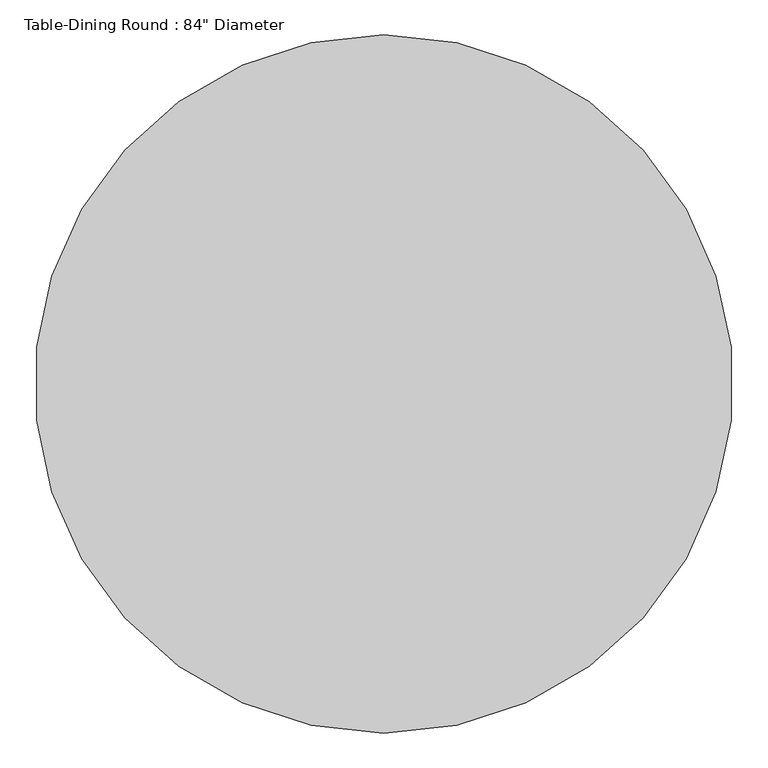
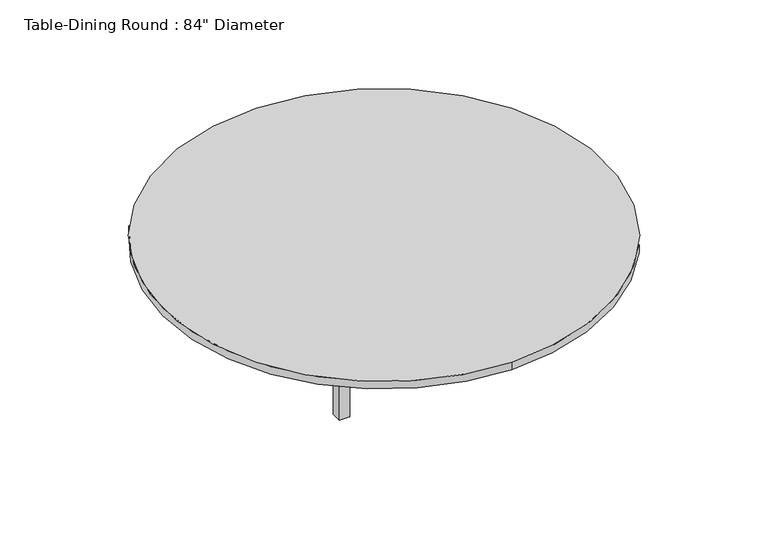
"""IFC4 building model written with IfcOpenShell, lengths in millimetres: furniture geometry."""

from ifc_helpers import new_model, si_unit, point, frame, frame_2d, origin, place, context, project, spatial, polyline, circle_curve, trimmed, segment, composite_curve, outline, extrude, faceted_brep, source, transform, mapped, element, save


def furniture_02b286f5(model_context):
    return source(origin(), model_context, "Body", "SolidModel", [
        extrude(outline(polyline([(637.0819672, 348.5213115), (637.0819672, -718.2786885), (-429.7180328, -718.2786885), (-429.7180328, 348.5213115), (637.0819672, 348.5213115)]), holes=[polyline([(611.6819672, 323.1213115), (-404.3180328, 323.1213115), (-404.3180328, -692.8786885), (611.6819672, -692.8786885), (611.6819672, 323.1213115)])]), frame((0.0, 0.0, 342.9), z_axis=(0.0, 0.0, 1.0), x_axis=(1.0, 0.0, 0.0)), (0.0, 0.0, 1.0), 76.2),
        faceted_brep([(-353.5180328, 323.1213115, 419.1), (-404.3180328, 323.1213115, 419.1), (-404.3180328, 272.3213115, 419.1), (-353.5180328, 272.3213115, 419.1), (560.8819672, 323.1213115, 419.1), (560.8819672, 272.3213115, 419.1), (611.6819672, 272.3213115, 419.1), (611.6819672, 323.1213115, 419.1), (560.8819672, -692.8786885, 419.1), (611.6819672, -692.8786885, 419.1), (611.6819672, -642.0786885, 419.1), (560.8819672, -642.0786885, 419.1), (-353.5180328, -692.8786885, 419.1), (-353.5180328, -642.0786885, 419.1), (-404.3180328, -642.0786885, 419.1), (-404.3180328, -692.8786885, 419.1), (-353.5180328, 323.1213115, 0.0), (-353.5180328, 272.3213115, 0.0), (-404.3180328, 272.3213115, 0.0), (-404.3180328, 323.1213115, 0.0), (560.8819672, 323.1213115, 0.0), (611.6819672, 323.1213115, 0.0), (611.6819672, 272.3213115, 0.0), (560.8819672, 272.3213115, 0.0), (560.8819672, -692.8786885, 0.0), (560.8819672, -642.0786885, 0.0), (611.6819672, -642.0786885, 0.0), (611.6819672, -692.8786885, 0.0), (-353.5180328, -692.8786885, 0.0), (-404.3180328, -692.8786885, 0.0), (-404.3180328, -642.0786885, 0.0), (-353.5180328, -642.0786885, 0.0), (-353.5180328, 323.1213115, 279.4), (560.8819672, 323.1213115, 279.4), (560.8819672, 323.1213115, 203.2), (-353.5180328, 323.1213115, 203.2), (560.8819672, 323.1213115, 228.6), (560.8819672, 323.1213115, 254.0), (-353.5180328, 323.1213115, 254.0), (-353.5180328, 323.1213115, 228.6), (-404.3180328, 272.3213115, 203.2), (-404.3180328, -642.0786885, 203.2), (-404.3180328, -642.0786885, 279.4), (-404.3180328, 272.3213115, 279.4), (-404.3180328, 272.3213115, 228.6), (-404.3180328, 272.3213115, 254.0), (-404.3180328, -642.0786885, 254.0), (-404.3180328, -642.0786885, 228.6), (-353.5180328, 272.3213115, 279.4), (-353.5180328, 272.3213115, 203.2), (-353.5180328, 272.3213115, 228.6), (-353.5180328, 272.3213115, 254.0), (560.8819672, 272.3213115, 279.4), (560.8819672, 272.3213115, 203.2), (560.8819672, 272.3213115, 228.6), (560.8819672, 272.3213115, 254.0), (611.6819672, 272.3213115, 279.4), (611.6819672, 272.3213115, 203.2), (611.6819672, 272.3213115, 228.6), (611.6819672, 272.3213115, 254.0), (611.6819672, -642.0786885, 279.4), (611.6819672, -642.0786885, 203.2), (611.6819672, -642.0786885, 228.6), (611.6819672, -642.0786885, 254.0), (560.8819672, -692.8786885, 279.4), (-353.5180328, -692.8786885, 279.4), (-353.5180328, -692.8786885, 203.2), (560.8819672, -692.8786885, 203.2), (-353.5180328, -692.8786885, 228.6), (-353.5180328, -692.8786885, 254.0), (560.8819672, -692.8786885, 254.0), (560.8819672, -692.8786885, 228.6), (560.8819672, -642.0786885, 279.4), (560.8819672, -642.0786885, 203.2), (560.8819672, -642.0786885, 228.6), (560.8819672, -642.0786885, 254.0), (-353.5180328, -642.0786885, 279.4), (-353.5180328, -642.0786885, 203.2), (-353.5180328, -642.0786885, 228.6), (-353.5180328, -642.0786885, 254.0)], [[[0, 1, 2, 3]], [[4, 5, 6, 7]], [[8, 9, 10, 11]], [[12, 13, 14, 15]], [[16, 17, 18, 19]], [[20, 21, 22, 23]], [[24, 25, 26, 27]], [[28, 29, 30, 31]], [[1, 0, 32, 33, 4, 7, 21, 20, 34, 35, 16, 19], [36, 37, 38, 39]], [[2, 1, 19, 18, 40, 41, 30, 29, 15, 14, 42, 43], [44, 45, 46, 47]], [[3, 2, 43, 48]], [[18, 17, 49, 40]], [[44, 50, 51, 45]], [[0, 3, 48, 32]], [[17, 16, 35, 49]], [[50, 39, 38, 51]], [[5, 4, 33, 52]], [[20, 23, 53, 34]], [[36, 54, 55, 37]], [[6, 5, 52, 56]], [[23, 22, 57, 53]], [[54, 58, 59, 55]], [[21, 7, 6, 56, 60, 10, 9, 27, 26, 61, 57, 22], [62, 63, 59, 58]], [[27, 9, 8, 64, 65, 12, 15, 29, 28, 66, 67, 24], [68, 69, 70, 71]], [[11, 10, 60, 72]], [[26, 25, 73, 61]], [[62, 74, 75, 63]], [[8, 11, 72, 64]], [[25, 24, 67, 73]], [[74, 71, 70, 75]], [[13, 12, 65, 76]], [[28, 31, 77, 66]], [[68, 78, 79, 69]], [[14, 13, 76, 42]], [[31, 30, 41, 77]], [[78, 47, 46, 79]], [[54, 74, 62, 58]], [[74, 78, 68, 71]], [[78, 50, 44, 47]], [[50, 54, 36, 39]], [[53, 49, 35, 34]], [[49, 77, 41, 40]], [[77, 73, 67, 66]], [[73, 53, 57, 61]], [[74, 54, 53, 73]], [[78, 74, 73, 77]], [[50, 78, 77, 49]], [[54, 50, 49, 53]], [[52, 72, 60, 56]], [[72, 76, 65, 64]], [[76, 48, 43, 42]], [[48, 52, 33, 32]], [[55, 51, 38, 37]], [[51, 79, 46, 45]], [[79, 75, 70, 69]], [[75, 55, 59, 63]], [[72, 52, 55, 75]], [[76, 72, 75, 79]], [[48, 76, 79, 51]], [[52, 48, 51, 55]]]),
        extrude(outline(composite_curve([segment(trimmed(circle_curve(frame_2d((103.6819672, -184.8786885)), 1066.8), [point((103.6819672, -1251.6786885))], [point((103.6819672, 881.9213115))], False, "CARTESIAN"), True, "CONTINUOUS"), segment(trimmed(circle_curve(frame_2d((103.6819672, -184.8786885)), 1066.8), [point((103.6819672, 881.9213115))], [point((103.6819672, -1251.6786885))], False, "CARTESIAN"), True, "CONTINUOUS")], self_intersect=False)), frame((0.0, 0.0, 419.1), z_axis=(0.0, 0.0, 1.0), x_axis=(1.0, 0.0, 0.0)), (0.0, 0.0, 1.0), 38.1),
    ])


if __name__ == "__main__":
    model = new_model("IFC4")
    model_context = context("Model", 3, world=origin())
    ifc_project = project(units=[si_unit("LENGTHUNIT", "METRE", prefix="MILLI")], contexts=[model_context])
    site = spatial("IfcSite", under=ifc_project)
    building = spatial("IfcBuilding", under=site)
    placement = place(None, origin())
    furniture_shape = furniture_02b286f5(model_context)
    element("IfcFurniture", 1, ObjectType="Table-Dining Round : 84\" Diameter", at=placement, inside=building, context=model_context, shape_type="MappedRepresentation", body=[
        mapped(furniture_shape, transform((0.0, 0.0, 0.0), x_axis=(1.0, 0.0, 0.0), y_axis=(0.0, 1.0, 0.0), z_axis=(0.0, 0.0, 1.0))),
    ])
    save(model, "model.ifc")

# Revit data of these elements
# Type "Table-Dining Round : 84\" Diameter"
#   Assembly Code = "E2020200"
#   Diameter = 7' - 0"
#   Height = 1' - 6"
#   Base Material = Pine
#   Top Material = Laminate, Linen, Matte
#   Default Elevation = 0
# Element 1 (IfcFurniture, "Table-Dining Round : 84\" Diameter")
#   Materials on its faces: "Pine", "Laminate, Linen, Matte"
# Materials
#   "Pine": class "Wood", colour RGB 223 192 134, transparency 0, Description = "Pinus Echinata", Cost = 0
#   "Laminate, Linen, Matte": class "Plastic", colour RGB 249 239 230, transparency 0, Description = "Plastic Laminate - Linen, Matte", Cost = 0
